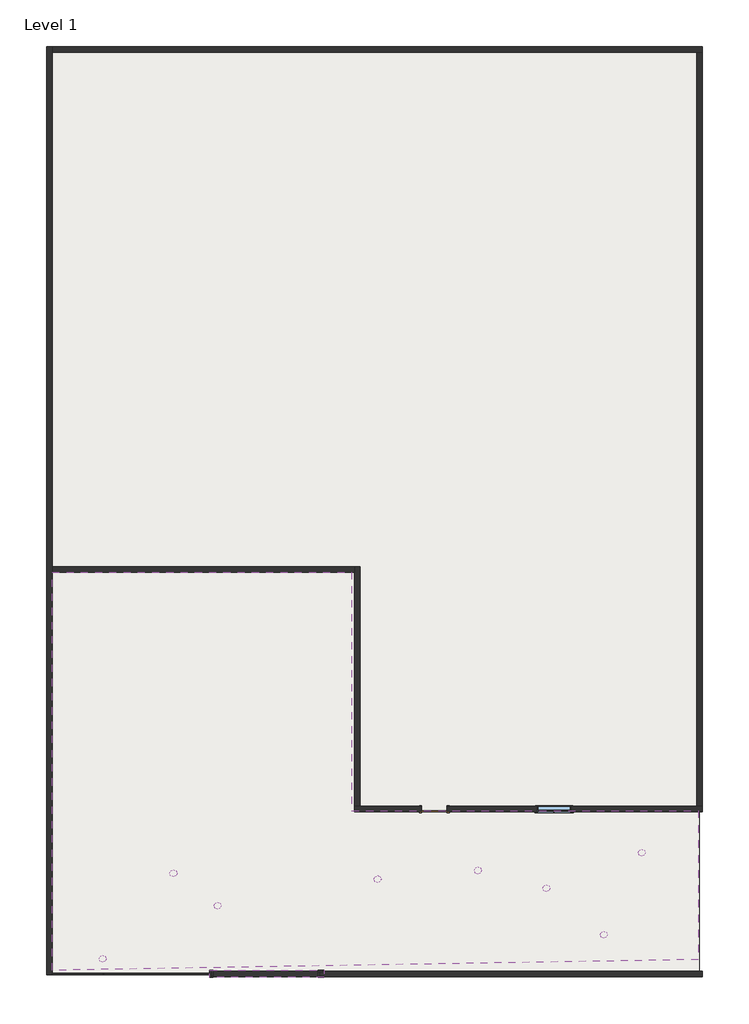
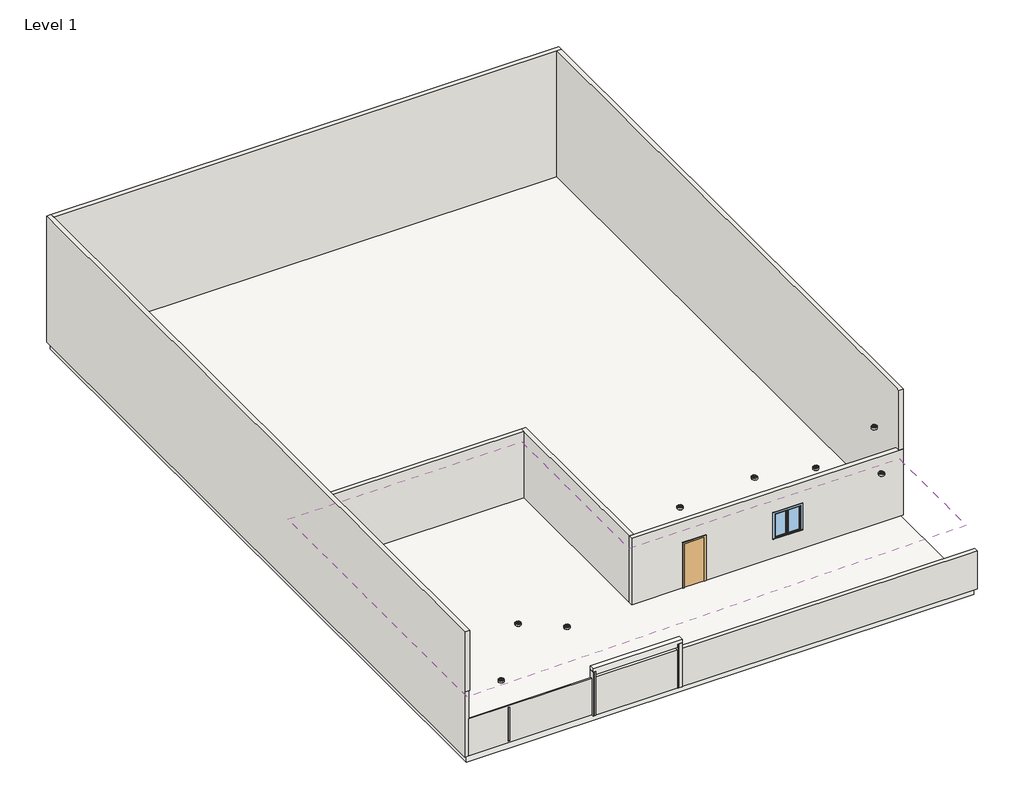
# One storey: 16 walls, 8 light fixtures, 2 slabs, 1 covering, 1 door, 1 window.
"""IFC4 building model written with IfcOpenShell, lengths in millimetres."""

from ifc_helpers import new_model, si_unit, frame, origin, origin_with_axes, place, context, project, spatial, polyline, outline, extrude, faceted_brep, transform, mapped, element, save
from components import door_54dd4da4, ceiling_light_flat_round_60w_120v_a3c1fe64, window_0862ab64

model = new_model("IFC4")

# Units and contexts
model_context = context("Model", 3, world=origin())
ifc_project = project(units=[si_unit("LENGTHUNIT", "METRE", prefix="MILLI")], contexts=[model_context])

# Site, building, storey
site = spatial("IfcSite", under=ifc_project)
building = spatial("IfcBuilding", under=site)
storey = spatial("IfcBuildingStorey", under=building, Name="Level 1", Elevation=0.0)

# Covering
placement = place(None, origin())
element("IfcCovering", 1, ObjectType="2' x 4' ACT System", at=placement, inside=storey, context=model_context, shape_type="SweptSolid", body=[
    extrude(outline(polyline([(-18299.5950104, -16741.3898918), (-18299.5950104, -2573.393541), (-7631.5950104, -2573.393541), (-7631.5950104, -11051.7898918), (4712.8049896, -11051.7898918), (4712.8049896, -16360.3898918), (-18299.5950104, -16741.3898918)])), frame((0.0, 0.0, 2743.2), z_axis=(0.0, 0.0, 1.0), x_axis=(1.0, 0.0, 0.0)), (0.0, 0.0, 1.0), 57.15),
])

# Door
door_shape = door_54dd4da4(model_context)
element("IfcDoor", 2, ObjectType="Single-Flush : 36\" x 84\"", at=placement, inside=storey, context=model_context, shape_type="MappedRepresentation", body=[
    mapped(door_shape, transform((-4685.1950104, -11000.9898918, 0.0), x_axis=(-1.0, 0.0, 0.0), y_axis=(0.0, -1.0, 0.0), z_axis=(0.0, 0.0, 1.0))),
])

# Light fixtures
ceiling_light_flat_round_60w_120v_shape = ceiling_light_flat_round_60w_120v_a3c1fe64(model_context)
element("IfcLightFixture", 3, ObjectType="Ceiling Light - Flat Round : 60W - 120V", at=placement, inside=storey, context=model_context, shape_type="MappedRepresentation", body=[
    mapped(ceiling_light_flat_round_60w_120v_shape, transform((-16507.9731231, -16334.248078, 2743.2), x_axis=(1.0, 0.0, 0.0), y_axis=(0.0, -1.0, 0.0), z_axis=(0.0, 0.0, -1.0))),
])
element("IfcLightFixture", 4, ObjectType="Ceiling Light - Flat Round : 60W - 120V", at=placement, inside=storey, context=model_context, shape_type="MappedRepresentation", body=[
    mapped(ceiling_light_flat_round_60w_120v_shape, transform((-12406.7950104, -14437.2971484, 2743.2), x_axis=(1.0, 0.0, 0.0), y_axis=(0.0, -1.0, 0.0), z_axis=(0.0, 0.0, -1.0))),
])
element("IfcLightFixture", 5, ObjectType="Ceiling Light - Flat Round : 60W - 120V", at=placement, inside=storey, context=model_context, shape_type="MappedRepresentation", body=[
    mapped(ceiling_light_flat_round_60w_120v_shape, transform((-13981.5950104, -13286.9898918, 2743.2), x_axis=(1.0, 0.0, 0.0), y_axis=(0.0, -1.0, 0.0), z_axis=(0.0, 0.0, -1.0))),
])
element("IfcLightFixture", 6, ObjectType="Ceiling Light - Flat Round : 60W - 120V", at=placement, inside=storey, context=model_context, shape_type="MappedRepresentation", body=[
    mapped(ceiling_light_flat_round_60w_120v_shape, transform((-6702.595824, -13492.8269449, 5943.6), x_axis=(1.0, 0.0, 0.0), y_axis=(0.0, -1.0, 0.0), z_axis=(0.0, 0.0, -1.0))),
])
element("IfcLightFixture", 7, ObjectType="Ceiling Light - Flat Round : 60W - 120V", at=placement, inside=storey, context=model_context, shape_type="MappedRepresentation", body=[
    mapped(ceiling_light_flat_round_60w_120v_shape, transform((-3135.7950104, -13187.9917164, 5943.6), x_axis=(1.0, 0.0, 0.0), y_axis=(0.0, -1.0, 0.0), z_axis=(0.0, 0.0, -1.0))),
])
element("IfcLightFixture", 8, ObjectType="Ceiling Light - Flat Round : 60W - 120V", at=placement, inside=storey, context=model_context, shape_type="MappedRepresentation", body=[
    mapped(ceiling_light_flat_round_60w_120v_shape, transform((1354.1459392, -15471.3898918, 5943.6), x_axis=(1.0, 0.0, 0.0), y_axis=(0.0, -1.0, 0.0), z_axis=(0.0, 0.0, -1.0))),
])
element("IfcLightFixture", 9, ObjectType="Ceiling Light - Flat Round : 60W - 120V", at=placement, inside=storey, context=model_context, shape_type="MappedRepresentation", body=[
    mapped(ceiling_light_flat_round_60w_120v_shape, transform((2706.2049896, -12550.3898918, 5943.6), x_axis=(1.0, 0.0, 0.0), y_axis=(0.0, -1.0, 0.0), z_axis=(0.0, 0.0, -1.0))),
])
element("IfcLightFixture", 10, ObjectType="Ceiling Light - Flat Round : 60W - 120V", at=placement, inside=storey, context=model_context, shape_type="MappedRepresentation", body=[
    mapped(ceiling_light_flat_round_60w_120v_shape, transform((-697.3950104, -13820.3898918, 5943.6), x_axis=(1.0, 0.0, 0.0), y_axis=(0.0, -1.0, 0.0), z_axis=(0.0, 0.0, -1.0))),
])

# Slabs
element("IfcSlab", 11, ObjectType="Generic - 12\"", at=placement, inside=storey, context=model_context, shape_type="SweptSolid", body=[
    extrude(outline(polyline([(4763.6049896, 16050.0101082), (4763.6049896, -16868.3898918), (-18401.1950104, -16868.3898918), (-18401.1950104, 16050.0101082), (4763.6049896, 16050.0101082)])), frame((0.0, 0.0, -304.8), z_axis=(0.0, 0.0, 1.0), x_axis=(1.0, 0.0, 0.0)), (0.0, 0.0, 1.0), 304.8),
])
element("IfcSlab", 12, ObjectType="Generic - 12\"", at=placement, inside=storey, context=model_context, shape_type="SweptSolid", body=[
    extrude(outline(polyline([(-8621.8916905, -16741.3898918), (-8621.8916905, -16995.3898918), (-12686.1950104, -16995.3898918), (-12686.1950104, -16741.3898918), (-8621.8916905, -16741.3898918)])), frame((0.0, 0.0, 1981.2), z_axis=(0.0, 0.0, 1.0), x_axis=(1.0, 0.0, 0.0)), (0.0, 0.0, 1.0), 304.8),
])

# Walls
element("IfcWall", 13, at=placement, inside=storey, context=model_context, shape_type="SweptSolid", body=[
    extrude(outline(polyline([(0.0, -18299.5950104), (0.0, -12686.1950104), (1778.5182319, -12686.1950104), (1778.5182319, -18299.5950104), (0.0, -18299.5950104)]), holes=[polyline([(1699.1786578, -16499.7617173), (1699.1786578, -16448.9617173), (73.5786578, -16448.9617173), (73.5786578, -16499.7617173), (1699.1786578, -16499.7617173)])]), frame((0.0, -16893.7898918, 0.0), z_axis=(0.0, 1.0, 0.0), x_axis=(0.0, 0.0, 1.0)), (0.0, 0.0, 1.0), 50.8),
])
element("IfcWall", 14, at=placement, inside=storey, context=model_context, shape_type="Brep", body=[
    faceted_brep([(-12686.1950104, -16792.1898918, 0.0), (-12635.3950104, -16792.1898918, 0.0), (-12615.0644202, -16792.1898918, 0.0), (-12615.0644202, -16792.1898918, 304.8), (-12635.3950104, -16792.1898918, 304.8), (-12686.1950104, -16792.1898918, 304.8), (-12686.1950104, -16741.3898918, 0.0), (-12686.1950104, -16741.3898918, 304.8), (-12615.0644202, -16741.3898918, 304.8), (-12615.0644202, -16741.3898918, 0.0), (-12686.1950104, -16766.7898918, 304.8)], [[[0, 1, 2, 3, 4, 5]], [[6, 7, 8, 9]], [[2, 1, 0, 6, 9]], [[5, 4, 3, 8, 7, 10]], [[0, 5, 10, 7, 6]], [[3, 2, 9, 8]]]),
])
element("IfcWall", 15, at=placement, inside=storey, context=model_context, shape_type="Brep", body=[
    faceted_brep([(-12635.3950104, -16995.3898918, 2133.6), (-12635.3950104, -16995.3898918, 0.0), (-12635.3950104, -16944.5898918, 0.0), (-12635.3950104, -16792.1898918, 0.0), (-12635.3950104, -16792.1898918, 304.8), (-12635.3950104, -16766.7898918, 304.8), (-12635.3950104, -16766.7898918, 2133.6), (-12635.3950104, -16944.5898918, 2133.6), (-12686.1950104, -16995.3898918, 0.0), (-12686.1950104, -16995.3898918, 2133.6), (-12686.1950104, -16766.7898918, 2133.6), (-12686.1950104, -16766.7898918, 304.8), (-12686.1950104, -16792.1898918, 304.8), (-12686.1950104, -16792.1898918, 0.0), (-12686.1950104, -16842.9898918, 0.0), (-12686.1950104, -16893.7898918, 0.0)], [[[0, 1, 2, 3, 4, 5, 6, 7]], [[8, 9, 10, 11, 12, 13, 14, 15]], [[3, 2, 1, 8, 15, 14, 13]], [[0, 7, 6, 10, 9]], [[0, 9, 8, 1]], [[11, 5, 4, 12]], [[4, 3, 13, 12]], [[6, 5, 11, 10]]]),
])
element("IfcWall", 16, at=placement, inside=storey, context=model_context, shape_type="Brep", body=[
    faceted_brep([(-12564.2644202, -16944.5898918, 0.0), (-12615.0644202, -16944.5898918, 0.0), (-12635.3950104, -16944.5898918, 0.0), (-12635.3950104, -16944.5898918, 2133.6), (-12615.0644202, -16944.5898918, 2133.6), (-12564.2644202, -16944.5898918, 2133.6), (-12564.2644202, -16995.3898918, 0.0), (-12564.2644202, -16995.3898918, 2133.6), (-12635.3950104, -16995.3898918, 2133.6), (-12635.3950104, -16995.3898918, 0.0)], [[[0, 1, 2, 3, 4, 5]], [[6, 7, 8, 9]], [[2, 1, 0, 6, 9]], [[5, 4, 3, 8, 7]], [[0, 5, 7, 6]], [[2, 9, 8, 3]]]),
])
element("IfcWall", 17, at=placement, inside=storey, context=model_context, shape_type="Brep", body=[
    faceted_brep([(-12615.0644202, -16741.3898918, 0.0), (-12615.0644202, -16792.1898918, 0.0), (-12615.0644202, -16944.5898918, 0.0), (-12615.0644202, -16944.5898918, 2133.6), (-12615.0644202, -16741.3898918, 2133.6), (-12615.0644202, -16741.3898918, 304.8), (-12564.2644202, -16741.3898918, 0.0), (-12564.2644202, -16741.3898918, 2133.6), (-12564.2644202, -16944.5898918, 2133.6), (-12564.2644202, -16944.5898918, 0.0)], [[[0, 1, 2, 3, 4, 5]], [[6, 7, 8, 9]], [[2, 1, 0, 6, 9]], [[4, 3, 8, 7]], [[0, 5, 4, 7, 6]], [[3, 2, 9, 8]]]),
])
element("IfcWall", 18, at=placement, inside=storey, context=model_context, shape_type="Brep", body=[
    faceted_brep([(-8829.5340594, -16792.1898918, 0.0), (-8778.7340594, -16792.1898918, 0.0), (-8672.6916905, -16792.1898918, 0.0), (-8672.6916905, -16792.1898918, 2133.6), (-8778.7340594, -16792.1898918, 2133.6), (-8829.5340594, -16792.1898918, 2133.6), (-8829.5340594, -16741.3898918, 0.0), (-8829.5340594, -16741.3898918, 2133.6), (-8672.6916905, -16741.3898918, 2133.6), (-8672.6916905, -16741.3898918, 304.8), (-8672.6916905, -16741.3898918, 0.0)], [[[0, 1, 2, 3, 4, 5]], [[6, 7, 8, 9, 10]], [[2, 1, 0, 6, 10]], [[5, 4, 3, 8, 7]], [[0, 5, 7, 6]], [[3, 2, 10, 9, 8]]]),
])
element("IfcWall", 19, at=placement, inside=storey, context=model_context, shape_type="Brep", body=[
    faceted_brep([(-8778.7340594, -16995.3898918, 0.0), (-8778.7340594, -16944.5898918, 0.0), (-8778.7340594, -16792.1898918, 0.0), (-8778.7340594, -16792.1898918, 2133.6), (-8778.7340594, -16944.5898918, 2133.6), (-8778.7340594, -16995.3898918, 2133.6), (-8829.5340594, -16995.3898918, 0.0), (-8829.5340594, -16995.3898918, 2133.6), (-8829.5340594, -16792.1898918, 2133.6), (-8829.5340594, -16792.1898918, 0.0)], [[[0, 1, 2, 3, 4, 5]], [[6, 7, 8, 9]], [[2, 1, 0, 6, 9]], [[5, 4, 3, 8, 7]], [[0, 5, 7, 6]], [[3, 2, 9, 8]]]),
])
element("IfcWall", 20, at=placement, inside=storey, context=model_context, shape_type="Brep", body=[
    faceted_brep([(-8621.8916905, -16944.5898918, 0.0), (-8672.6916905, -16944.5898918, 0.0), (-8778.7340594, -16944.5898918, 0.0), (-8778.7340594, -16944.5898918, 2133.6), (-8621.8916905, -16944.5898918, 2133.6), (-8621.8916905, -16944.5898918, 304.8), (-8621.8916905, -16995.3898918, 0.0), (-8621.8916905, -16995.3898918, 2133.6), (-8778.7340594, -16995.3898918, 2133.6), (-8778.7340594, -16995.3898918, 0.0)], [[[0, 1, 2, 3, 4, 5]], [[6, 7, 8, 9]], [[2, 1, 0, 6, 9]], [[4, 3, 8, 7]], [[0, 5, 4, 7, 6]], [[3, 2, 9, 8]]]),
])
element("IfcWall", 21, at=placement, inside=storey, context=model_context, shape_type="Brep", body=[
    faceted_brep([(-8672.6916905, -16741.3898918, 0.0), (-8672.6916905, -16792.1898918, 0.0), (-8672.6916905, -16944.5898918, 0.0), (-8672.6916905, -16944.5898918, 304.8), (-8672.6916905, -16741.3898918, 304.8), (-8621.8916905, -16741.3898918, 0.0), (-8621.8916905, -16741.3898918, 304.8), (-8621.8916905, -16944.5898918, 304.8), (-8621.8916905, -16944.5898918, 0.0)], [[[0, 1, 2, 3, 4]], [[5, 6, 7, 8]], [[2, 1, 0, 5, 8]], [[4, 3, 7, 6]], [[0, 4, 6, 5]], [[3, 2, 8, 7]]]),
])
element("IfcWall", 22, ObjectType="Generic - 8\"", at=placement, inside=storey, context=model_context, shape_type="Brep", body=[
    faceted_brep([(-5142.3950104, -10899.3898918, 2133.6), (-5142.3950104, -10899.3898918, 0.0), (-7326.7950104, -10899.3898918, 0.0), (-7529.9950104, -10899.3898918, 0.0), (-7529.9950104, -10899.3898918, 3200.4), (-7326.7950104, -10899.3898918, 3200.4), (4662.0049896, -10899.3898918, 3200.4), (4865.2049896, -10899.3898918, 3200.4), (4865.2049896, -10899.3898918, 0.0), (4662.0049896, -10899.3898918, 0.0), (-4227.9950104, -10899.3898918, 0.0), (-4227.9950104, -10899.3898918, 2133.6), (-1027.5950104, -10899.3898918, 2133.6), (-1027.5950104, -10899.3898918, 914.4), (191.6049896, -10899.3898918, 914.4), (191.6049896, -10899.3898918, 2133.6), (-7529.9950104, -11102.5898918, 0.0), (-5142.3950104, -11102.5898918, 0.0), (-5142.3950104, -11102.5898918, 2133.6), (-4227.9950104, -11102.5898918, 2133.6), (-4227.9950104, -11102.5898918, 0.0), (4865.2049896, -11102.5898918, 0.0), (4865.2049896, -11102.5898918, 3200.4), (4662.0049896, -11102.5898918, 3200.4), (-7529.9950104, -11102.5898918, 3200.4), (-1027.5950104, -11102.5898918, 2133.6), (191.6049896, -11102.5898918, 2133.6), (191.6049896, -11102.5898918, 914.4), (-1027.5950104, -11102.5898918, 914.4)], [[[0, 1, 2, 3, 4, 5, 6, 7, 8, 9, 10, 11], [12, 13, 14, 15]], [[16, 17, 18, 19, 20, 21, 22, 23, 24], [25, 26, 27, 28]], [[10, 9, 8, 21, 20]], [[3, 2, 1, 17, 16]], [[7, 6, 5, 4, 24, 23, 22]], [[4, 3, 16, 24]], [[8, 7, 22, 21]], [[18, 17, 1, 0]], [[19, 18, 0, 11]], [[20, 19, 11, 10]], [[13, 12, 25, 28]], [[14, 13, 28, 27]], [[15, 14, 27, 26]], [[12, 15, 26, 25]]]),
])
element("IfcWall", 23, ObjectType="Generic - 8\"", at=placement, inside=storey, context=model_context, shape_type="Brep", body=[
    faceted_brep([(-7326.7950104, -10899.3898918, 0.0), (-7326.7950104, -2370.193541, 0.0), (-7326.7950104, -2370.193541, 3200.4), (-7326.7950104, -10899.3898918, 3200.4), (-7529.9950104, -10899.3898918, 0.0), (-7529.9950104, -10899.3898918, 3200.4), (-7529.9950104, -2573.393541, 3200.4), (-7529.9950104, -2370.193541, 3200.4), (-7529.9950104, -2370.193541, 0.0), (-7529.9950104, -2573.393541, 0.0)], [[[0, 1, 2, 3]], [[4, 5, 6, 7, 8, 9]], [[1, 0, 4, 9, 8]], [[3, 2, 7, 6, 5]], [[0, 3, 5, 4]], [[2, 1, 8, 7]]]),
])
element("IfcWall", 24, ObjectType="Generic - 8\"", at=placement, inside=storey, context=model_context, shape_type="SweptSolid", body=[
    extrude(outline(polyline([(-18299.5950104, -2370.193541), (-7529.9950104, -2370.193541), (-7529.9950104, -2573.393541), (-18299.5950104, -2573.393541), (-18299.5950104, -2370.193541)])), origin_with_axes(), (0.0, 0.0, 1.0), 3200.4),
])
element("IfcWall", 25, ObjectType="Generic - 8\"", at=placement, inside=storey, context=model_context, shape_type="Brep", body=[
    faceted_brep([(-18299.5950104, 15948.4101082, 0.0), (4662.0049896, 15948.4101082, 0.0), (4865.2049896, 15948.4101082, 0.0), (4865.2049896, 15948.4101082, 6096.0), (4662.0049896, 15948.4101082, 6096.0), (-18299.5950104, 15948.4101082, 6096.0), (-18299.5950104, 16151.6101082, 0.0), (-18299.5950104, 16151.6101082, 6096.0), (4865.2049896, 16151.6101082, 6096.0), (4865.2049896, 16151.6101082, 0.0)], [[[0, 1, 2, 3, 4, 5]], [[6, 7, 8, 9]], [[2, 1, 0, 6, 9]], [[5, 4, 3, 8, 7]], [[0, 5, 7, 6]], [[3, 2, 9, 8]]]),
])
element("IfcWall", 26, ObjectType="Generic - 8\"", at=placement, inside=storey, context=model_context, shape_type="Brep", body=[
    faceted_brep([(4662.0049896, 15948.4101082, 0.0), (4662.0049896, -10899.3898918, 0.0), (4662.0049896, -10899.3898918, 3200.4), (4662.0049896, -11102.5898918, 3200.4), (4662.0049896, -11102.5898918, 6096.0), (4662.0049896, -10899.3898918, 6096.0), (4662.0049896, 15948.4101082, 6096.0), (4865.2049896, 15948.4101082, 0.0), (4865.2049896, 15948.4101082, 6096.0), (4865.2049896, -11102.5898918, 6096.0), (4865.2049896, -11102.5898918, 3200.4), (4865.2049896, -10899.3898918, 3200.4), (4865.2049896, -10899.3898918, 0.0), (4763.6049896, -11102.5898918, 3200.4)], [[[0, 1, 2, 3, 4, 5, 6]], [[7, 8, 9, 10, 11, 12]], [[1, 0, 7, 12]], [[6, 5, 4, 9, 8]], [[0, 6, 8, 7]], [[10, 13, 3, 2, 11]], [[2, 1, 12, 11]], [[4, 3, 13, 10, 9]]]),
])
element("IfcWall", 27, ObjectType="Generic - 8\"", at=placement, inside=storey, context=model_context, shape_type="SweptSolid", body=[
    extrude(outline(polyline([(-12660.7950104, -16766.7898918), (4865.2049896, -16766.7898918), (4865.2049896, -16969.9898918), (-12660.7950104, -16969.9898918), (-12660.7950104, -16766.7898918)])), origin_with_axes(), (0.0, 0.0, 1.0), 1828.8),
])
element("IfcWall", 28, ObjectType="side wall", at=placement, inside=storey, context=model_context, shape_type="Brep", body=[
    faceted_brep([(-18299.5950104, -16893.7898918, 0.0), (-18299.5950104, -16842.9898918, 0.0), (-18299.5950104, -2573.393541, 0.0), (-18299.5950104, -2370.193541, 0.0), (-18299.5950104, 15948.4101082, 0.0), (-18299.5950104, 16151.6101082, 0.0), (-18299.5950104, 16151.6101082, 6096.0), (-18299.5950104, 15948.4101082, 6096.0), (-18299.5950104, -16969.9898918, 6096.0), (-18299.5950104, -16969.9898918, 3200.4), (-18299.5950104, -16893.7898918, 3200.4), (-18299.5950104, -16893.7898918, 1778.5182319), (-18502.7950104, -16893.7898918, 0.0), (-18502.7950104, -16893.7898918, 3200.4), (-18502.7950104, -16969.9898918, 3200.4), (-18502.7950104, -16969.9898918, 6096.0), (-18502.7950104, 16151.6101082, 6096.0), (-18502.7950104, 16151.6101082, 0.0)], [[[0, 1, 2, 3, 4, 5, 6, 7, 8, 9, 10, 11]], [[12, 13, 14, 15, 16, 17]], [[5, 4, 3, 2, 1, 0, 12, 17]], [[8, 7, 6, 16, 15]], [[6, 5, 17, 16]], [[9, 14, 13, 10]], [[0, 11, 10, 13, 12]], [[9, 8, 15, 14]]]),
])

# Window
window_shape = window_0862ab64(model_context)
element("IfcWindow", 29, ObjectType="Casement Dbl with Trim : 48\" x 48\"", at=placement, inside=storey, context=model_context, shape_type="MappedRepresentation", body=[
    mapped(window_shape, transform((-417.9950104, -10981.9398918, 0.0), x_axis=(-1.0, 0.0, 0.0), y_axis=(0.0, -1.0, 0.0), z_axis=(0.0, 0.0, 1.0))),
])

save(model, "model.ifc")

# Revit data of these elements
# Type "2' x 4' ACT System"
#   Assembly Code = "C3030210"
#   built-in parameter 1002203 = 1 (stored number, unit not read)
#   built-in parameter 1002202 = 1 (stored number, unit not read)
#   Layers, outside or top first: 0' - 1 5/8" "Default" (function 1); 0' - 0 5/8" "Acoustic Ceiling Tile 24 x 48" (function 5)
# Type "Single-Flush : 36\" x 84\""
#   Type Mark = "1"
#   Construction Type Id = "MDOOR"
#   Assembly Code = "C1020"
#   Analytic Construction = "Metal"
#   Thickness = 0' - 2"
#   Heat Transfer Coefficient (U) = 0.651978 BTU/(h·ft²·°F)
#   Height = 7' - 0"
#   Trim Projection Ext = 0' - 1"
#   Trim Projection Int = 0' - 1"
#   Trim Width = 0' - 3"
#   Width = 3' - 0"
#   Define Thermal Properties by = 1
#   Door Material = Door - Panel
#   Frame Material = Door - Frame
#   Visual Light Transmittance = 0
#   Solar Heat Gain Coefficient = 0
#   Function = (empty or 0)
#   Wall Closure = (empty or 0)
# Type "Ceiling Light - Flat Round : 60W - 120V"
#   Lamp = "A-19"
#   Photometric Web File = "CLFR1A19.ies"
#   Assembly Code = "D5020220"
#   Wattage = 60 W
#   built-in parameter 1150110 = 1 (stored number, unit not read)
#   built-in parameter 1150109 = 1 (stored number, unit not read)
#   built-in parameter 1150113 = 1 (stored number, unit not read)
#   Tilt Angle = -90.00°
#   built-in parameter 1150115 = 1 (stored number, unit not read)
#   built-in parameter 1150105 = 68.0387 (stored number, unit not read)
#   built-in parameter 1150112 = 1 (stored number, unit not read)
#   built-in parameter 1150114 = 1 (stored number, unit not read)
#   built-in parameter 1150107 = 2800 (stored number, unit not read)
#   built-in parameter 1150106 = 0.680387 (stored number, unit not read)
#   Emit from Circle Diameter = 0' - 10"
#   built-in parameter 1150104 = 1.32387 (stored number, unit not read)
#   Lumens = 855 lm
#   built-in parameter 1114217 = 1 (stored number, unit not read)
#   Default Elevation = 4' - 0"
#   Ballast Voltage = 120 V
#   built-in parameter 1114218 = 1 (stored number, unit not read)
#   built-in parameter 1150133 = 10 (stored number, unit not read)
#   Apparent Load = 60 VA
#   built-in parameter 1150134 = 4
#   built-in parameter 1150137 = 1
#   Color Filter = 16777215
#   built-in parameter 1140040 [instance default] = 1
#   Ballast Number of Poles = 1
#   Light Box Material = Steel, Paint Finish, Dark Gray, Matte
#   Diffuser Material = Glass, White, High Luminance
#   Emit Shape Visible in Rendering = no
#   Dimming Lamp Color Temperature Shift = (empty or 0)
# Type "Generic - 12\""
#   Assembly Code = "B1010"
#   Function = 0
#   Layers, outside or top first: 1' - 0" no material (function 1)
# Type
#   Assembly Code = "B2010"
#   Layers, outside or top first: 0' - 1 1/2" "Softwood, Lumber" (function 1); 0' - 0 1/2" "Door - Frame" (function 5)
# Type "Generic - 8\""
#   Assembly Code = "B2010"
#   Layers, outside or top first: 0' - 8" no material (function 1)
# Type "side wall"
#   Assembly Code = "B2010"
#   Layers, outside or top first: 0' - 8" "Sash" (function 1)
# Type "Casement Dbl with Trim : 48\" x 48\""
#   Type Mark = "19"
#   Construction Type Id = "GSP4R"
#   Assembly Code = "B2020100"
#   Analytic Construction = "1/8 in Pilkington single glazing"
#   Visual Light Transmittance = 0.9
#   Solar Heat Gain Coefficient = 0.78
#   Heat Transfer Coefficient (U) = 0.6496 BTU/(h·ft²·°F)
#   Height = 4' - 0"
#   Default Sill Height = 3' - 0"
#   Trim Projection - Ext. = 0' - 0 1/2"
#   Trim Projection - Int. = 0' - 0 3/4"
#   Trim Width - Exterior = 0' - 3 1/2"
#   Trim Width - Interior = 0' - 3 1/2"
#   Width = 4' - 0"
#   Window Inset = 0' - 0 3/4"
#   Define Thermal Properties by = 1
#   Glass Pane Material = Glass
#   Sash Material = Sash
#   Trim Exterior Material = Trim
#   Trim Interior Material = Trim
#   Wall Closure = (empty or 0)
# Element 1 (IfcCovering, "2' x 4' ACT System")
#   Height Offset From Level = 9' - 0"
#   Phase Created = New Construction
#   Materials on its faces: "Acoustic Ceiling Tile 24 x 48", "Default"
# Element 2 (IfcDoor, "Single-Flush : 36\" x 84\"")
#   Phase Created = New Construction
#   Materials on its faces: "Door - Frame", "Door - Panel"
# Element 3 (IfcLightFixture, "Ceiling Light - Flat Round : 60W - 120V")
#   Mark = "1"
#   built-in parameter 1140040 = 1
#   Phase Created = New Construction
#   Materials on its faces: "Glass, White, High Luminance", "Steel, Paint Finish, Dark Gray, Matte"
# Element 4 (IfcLightFixture, "Ceiling Light - Flat Round : 60W - 120V")
#   Mark = "2"
#   built-in parameter 1140040 = 1
#   Phase Created = New Construction
#   Materials on its faces: "Glass, White, High Luminance", "Steel, Paint Finish, Dark Gray, Matte"
# Element 5 (IfcLightFixture, "Ceiling Light - Flat Round : 60W - 120V")
#   Mark = "3"
#   built-in parameter 1140040 = 1
#   Phase Created = New Construction
#   Materials on its faces: "Glass, White, High Luminance", "Steel, Paint Finish, Dark Gray, Matte"
# Element 6 (IfcLightFixture, "Ceiling Light - Flat Round : 60W - 120V")
#   Mark = "4"
#   built-in parameter 1140040 = 1
#   Phase Created = New Construction
#   Materials on its faces: "Glass, White, High Luminance", "Steel, Paint Finish, Dark Gray, Matte"
# Element 7 (IfcLightFixture, "Ceiling Light - Flat Round : 60W - 120V")
#   Mark = "5"
#   built-in parameter 1140040 = 1
#   Phase Created = New Construction
#   Materials on its faces: "Glass, White, High Luminance", "Steel, Paint Finish, Dark Gray, Matte"
# Element 8 (IfcLightFixture, "Ceiling Light - Flat Round : 60W - 120V")
#   Mark = "6"
#   built-in parameter 1140040 = 1
#   Phase Created = New Construction
#   Materials on its faces: "Glass, White, High Luminance", "Steel, Paint Finish, Dark Gray, Matte"
# Element 9 (IfcLightFixture, "Ceiling Light - Flat Round : 60W - 120V")
#   Mark = "7"
#   built-in parameter 1140040 = 1
#   Phase Created = New Construction
#   Materials on its faces: "Glass, White, High Luminance", "Steel, Paint Finish, Dark Gray, Matte"
# Element 10 (IfcLightFixture, "Ceiling Light - Flat Round : 60W - 120V")
#   Mark = "8"
#   built-in parameter 1140040 = 1
#   Phase Created = New Construction
#   Materials on its faces: "Glass, White, High Luminance", "Steel, Paint Finish, Dark Gray, Matte"
# Element 11 (IfcSlab, "Generic - 12\"")
#   Height Offset From Level = 0' - 0"
#   Phase Created = New Construction
#   Materials on its faces: "Default Floor"
# Element 12 (IfcSlab, "Generic - 12\"")
#   Height Offset From Level = 7' - 6"
#   Phase Created = New Construction
#   Materials on its faces: "Default Floor"
# Element 13 (IfcWall)
#   Top Offset = 0' - 0"
#   Base Offset = 0' - 0"
#   Unconnected Height = 5' - 10.0204"
#   wall height = 5' - 10.0204"
#   Phase Created = New Construction
#   Base Constraint = Level 1
#   Materials on its faces: "Default Wall", "Door - Frame", "Softwood, Lumber"
# Elements 14, 21 (IfcWall)
#   Top Offset = 0' - 0"
#   Base Offset = 0' - 0"
#   Unconnected Height = 1' - 0"
#   wall height = 1' - 0"
#   Phase Created = New Construction
#   Base Constraint = Level 1
#   Materials on its faces: "Default Wall", "Softwood, Lumber", "Door - Frame"
# Elements 15, 16, 17, 18, 19, 20 (IfcWall)
#   Top Offset = 0' - 0"
#   Base Offset = 0' - 0"
#   Unconnected Height = 7' - 0"
#   wall height = 7' - 0"
#   Phase Created = New Construction
#   Base Constraint = Level 1
#   Materials on its faces: "Default Wall", "Softwood, Lumber", "Door - Frame"
# Elements 22, 23, 24 (IfcWall, "Generic - 8\"")
#   Top Offset = 0' - 0"
#   Base Offset = 0' - 0"
#   Unconnected Height = 10' - 6"
#   wall height = 10' - 6"
#   Phase Created = New Construction
#   Base Constraint = Level 1
#   Materials on its faces: "Default Wall"
# Element 25 (IfcWall, "Generic - 8\"")
#   Top Offset = 0' - 0"
#   Base Offset = 0' - 0"
#   Unconnected Height = 20' - 0"
#   wall height = 20' - 0"
#   Phase Created = New Construction
#   Base Constraint = Level 1
#   Materials on its faces: "Default Wall"
# Element 26 (IfcWall, "Generic - 8\"")
#   Top Offset = 0' - 0"
#   Base Offset = 0' - 0"
#   Unconnected Height = 20' - 0"
#   wall height = 20' - 0"
#   Phase Created = New Construction
#   Base Constraint = Level 1
#   Materials on its faces: "Default Wall", "Sash"
# Element 27 (IfcWall, "Generic - 8\"")
#   Top Offset = 0' - 0"
#   Base Offset = 0' - 0"
#   Unconnected Height = 6' - 0"
#   wall height = 6' - 0"
#   Phase Created = New Construction
#   Base Constraint = Level 1
#   Materials on its faces: "Default Wall"
# Element 28 (IfcWall, "side wall")
#   Top Offset = 0' - 0"
#   Base Offset = 0' - 0"
#   Unconnected Height = 20' - 0"
#   wall height = 20' - 0"
#   Phase Created = New Construction
#   Base Constraint = Level 1
#   Materials on its faces: "Sash", "Default Wall", "Door - Frame"
# Element 29 (IfcWindow, "Casement Dbl with Trim : 48\" x 48\"")
#   Mark = "1"
#   Phase Created = New Construction
#   Materials on its faces: "Sash", "Trim", "Glass"
# Materials
#   "Default": colour RGB 127 127 127, transparency 0
#   "Acoustic Ceiling Tile 24 x 48": class "Generic", colour RGB 229 229 229, transparency 0, Description = "Acoustic Ceiling Tile 24 x 48", Cost = 0
#   "Door - Panel": class "Wood", colour RGB 210 159 95, transparency 0
#   "Door - Frame": colour RGB 118 70 51, transparency 0
#   "Steel, Paint Finish, Dark Gray, Matte": class "Metal", colour RGB 98 98 98, transparency 0, Description = "Steel, paint finish, dark gray, matte", Cost = 0
#   "Glass, White, High Luminance": class "Glass", colour RGB 249 250 249, transparency 0.8, Description = "physical material", Cost = 0
#   "Softwood, Lumber": class "Wood", colour RGB 223 192 134, transparency 0, Description = "Pinus Echinata", Cost = 0
#   "Sash": class "Wood", colour RGB 255 255 255, transparency 0, Cost = 0
#   "Glass": class "Glass", colour RGB 0 128 192, transparency 0.75, Description = "Soda Lime Glass", Cost = 0
#   "Trim": class "Wood", colour RGB 224 178 126, transparency 0
#   "Default Floor": colour RGB 128 128 128, transparency 0
#   "Default Wall": colour RGB 128 128 128, transparency 0
